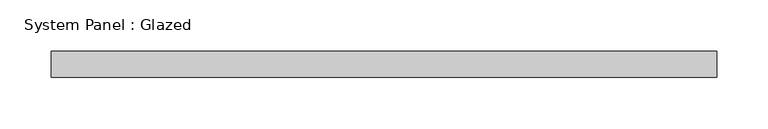
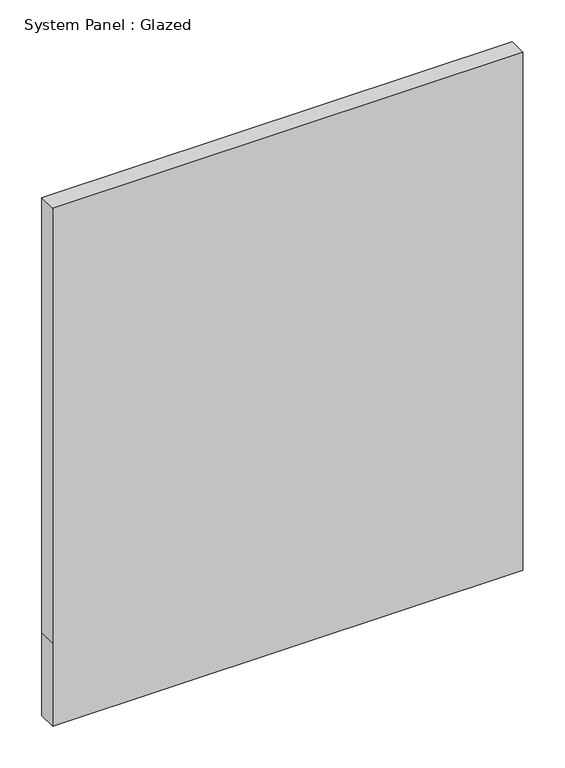
"""IFC4 building model written with IfcOpenShell, lengths in millimetres: plate geometry, System Panel : Glazed."""

from ifc_helpers import new_model, si_unit, frame, origin, place, context, project, spatial, polyline, outline, extrude, source, transform, mapped, element, save


def system_panel_glazed_5b2e8898(model_context):
    return source(origin(), model_context, "Body", "SweptSolid", [
        extrude(outline(polyline([(0.0, -323.85), (0.0, 323.85), (120.65, 323.85), (754.0943895, 323.85), (754.0943895, -323.85), (120.65, -323.85), (0.0, -323.85)])), frame((0.0, 19.05, 0.0), z_axis=(0.0, 1.0, 0.0), x_axis=(0.0, 0.0, 1.0)), (0.0, 0.0, 1.0), 25.4),
    ])


if __name__ == "__main__":
    model = new_model("IFC4")
    model_context = context("Model", 3, world=origin())
    ifc_project = project(units=[si_unit("LENGTHUNIT", "METRE", prefix="MILLI")], contexts=[model_context])
    site = spatial("IfcSite", under=ifc_project)
    building = spatial("IfcBuilding", under=site)
    placement = place(None, origin())
    system_panel_glazed_shape = system_panel_glazed_5b2e8898(model_context)
    element("IfcPlate", 1, ObjectType="System Panel : Glazed", at=placement, inside=building, context=model_context, shape_type="MappedRepresentation", body=[
        mapped(system_panel_glazed_shape, transform((0.0, 0.0, 0.0), x_axis=(1.0, 0.0, 0.0), y_axis=(0.0, 1.0, 0.0), z_axis=(0.0, 0.0, 1.0))),
    ])
    save(model, "model.ifc")

# Revit data of these elements
# Type "System Panel : Glazed"
#   Construction Type Id = "GSP4R"
#   Analytic Construction = "1/8 in Pilkington single glazing"
#   Visual Light Transmittance = 0.9
#   Solar Heat Gain Coefficient = 0.86
#   Heat Transfer Coefficient (U) = 1.18115 BTU/(h·ft²·°F)
#   Define Thermal Properties by = 1
# Element 1 (IfcPlate, "System Panel : Glazed")
#   Materials on its faces: "Glass"
# Materials
#   "Glass": class "Glass", colour RGB 0 128 192, transparency 0.75, Description = "Soda Lime Glass", Cost = 0
